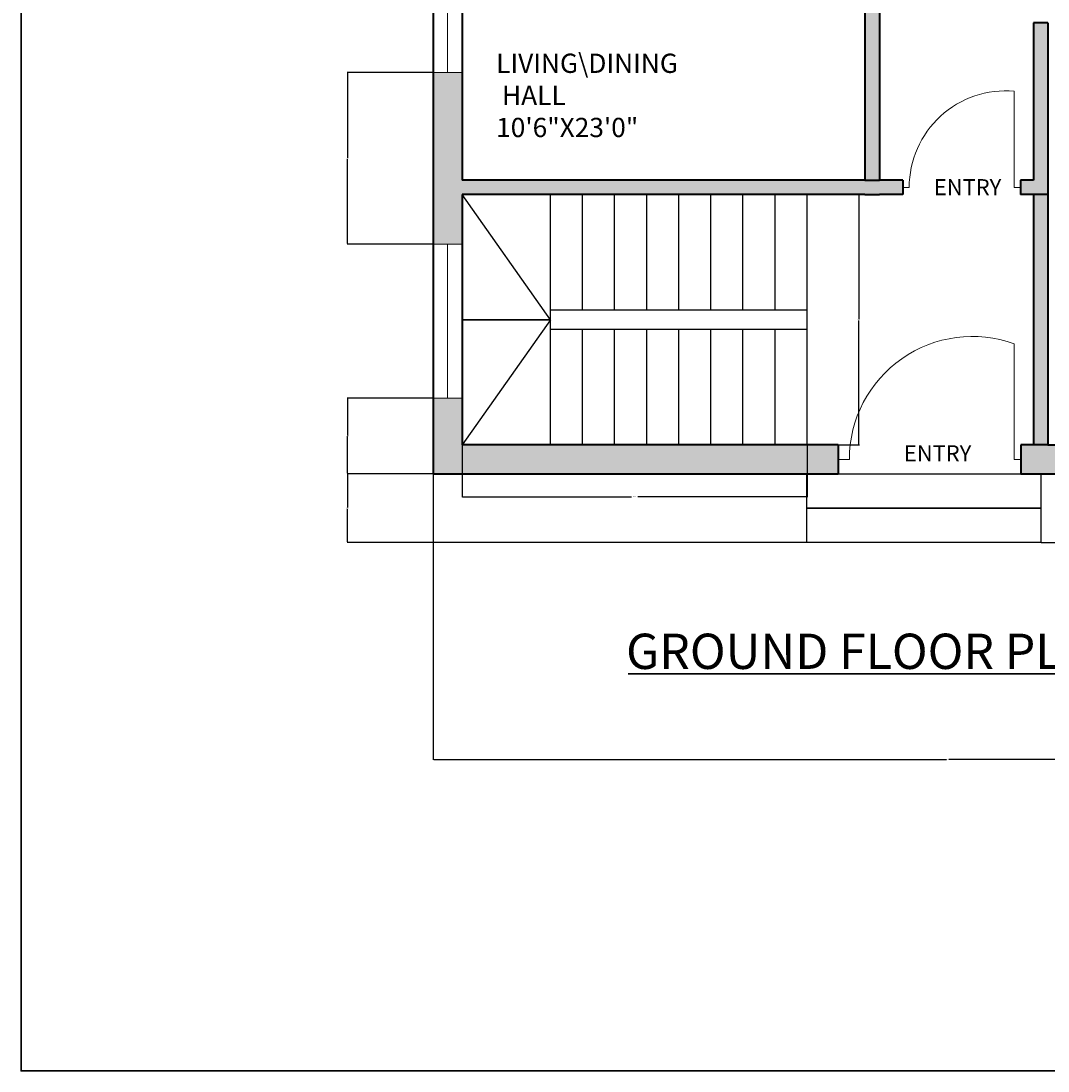
# Model space of a CAD drawing. Units: inches. Extents: x 1441 to 2460, y 1648 to 2683.
# Tile 1 of 35: x 1441 to 1760, y 1648 to 1975. Entities that reach past the tile are written whole.
import ezdxf

# ---------------------------------------------------------------- set-up
doc = ezdxf.new("R2010")
doc.units = ezdxf.units.IN
for name, color, linetype, lineweight in [('A-ANNO-DIMS', 2, 'Continuous', 18), ('A-ANNO-TEXT', 7, 'Continuous', 18), ('A-ANNO-TITL', 7, 'Continuous', 30), ('A-ANNO-TTLB', 7, 'Continuous', 35), ('A-AREA-IDEN', 7, 'Continuous', 20), ('A-DOOR', 3, 'Continuous', 20), ('A-FLOR-STRS', 7, 'Continuous', 25), ('A-GLAZ', 4, 'Continuous', 18), ('A-WALL', 7, 'Continuous', 40)]:
    doc.layers.add(name, color=color, linetype=linetype, lineweight=lineweight)
doc.layers.add('A-WALL-PATT', color=251, linetype='Continuous', lineweight=13, true_color=0x636466)
doc.styles.get("Standard").update_dxf_attribs({"font": 'arial.ttf'})
doc.dimstyles.get("Standard").update_dxf_attribs({"dimtxt": 0.18, "dimasz": 0.18, "dimexe": 0.18, "dimexo": 0.0625, "dimgap": 0.09, "dimtad": 0, "dimtih": 1, "dimtoh": 1, "dimdec": 4, "dimzin": 0, "dimdsep": 46, "dimtxsty": 'Standard', "dimcen": 0.09, "dimadec": 0, "dimazin": 0, "dimtfac": 1, "dimtdec": 4, "dimtofl": 0, "dimtmove": 0, "dimatfit": 3, "dimfxl": 1, "dimtolj": 1, "dimtzin": 0, "dimarcsym": 0})

# ---------------------------------------------------------------- blocks, each defined once
blk = doc.blocks.new('DOOR-ENTRY-OUTER')
for p, q in [((54.89, 0), (54.89, 36)), ((0, 0), (1.52, 0)), ((1.52, 0), (3.52, 0)), ((56.89, 0), (54.89, 0))]:
    blk.add_line(p, q)
blk.add_arc((41.82, 0), 38.3, 70.0399, 180)
blk = doc.blocks.new('DOOR-ENTRY-INNER')
for p, q in [((34.71, 24.01), (34.71, 30.01)), ((34.71, 0.01), (34.71, 24.01)), ((0, 0.01), (2, 0.01)), ((36.71, 0.01), (34.71, 0.01))]:
    blk.add_line(p, q)
blk.add_arc((32.11, 0.01), 30.11, 85.0485, 180)
blk = doc.blocks.new('WIN-48-SASH')
for p, q in [((9, 48), (4.5, 48)), ((4.5, 48), (4.5, 0)), ((4.5, 0), (0, 0))]:
    blk.add_line(p, q)
blk = doc.blocks.new('STAIR-RETURN-PLAN')
for p, q in [((27.5, 39), (0, 78)), ((27.5, 0), (27.5, 78)), ((37.5, 42), (37.5, 78)), ((47.5, 42), (47.5, 78)), ((57.5, 42), (57.5, 78)), ((67.5, 42), (67.5, 78)), ((77.5, 42), (77.5, 78)), ((87.5, 42), (87.5, 78)), ((97.5, 42), (97.5, 78)), ((107.5, 0), (107.5, 78)), ((107.5, 42), (27.5, 42)), ((27.5, 39), (0, 39)), ((0, 39), (27.5, 39)), ((27.5, 39), (0, 0)), ((107.5, 36), (27.5, 36)), ((37.5, 0), (37.5, 36)), ((47.5, 0), (47.5, 36)), ((57.5, 0), (57.5, 36)), ((67.5, 0), (67.5, 36)), ((77.5, 0), (77.5, 36)), ((87.5, 0), (87.5, 36)), ((97.5, 0), (97.5, 36))]:
    blk.add_line(p, q)
blk = doc.blocks.new('*D40')
at = {"layer": 'A-ANNO-DIMS', "color": 0, "lineweight": -2, "transparency": 16777216}
for p, q in [((1577.89, 1843.13), (1577.89, 1826.89)), ((1685.39, 1843.13), (1685.39, 1826.89)), ((1578.07, 1827.07), (1630.64, 1827.07)), ((1685.21, 1827.07), (1632.64, 1827.07))]:
    blk.add_line(p, q, dxfattribs=at)
at = {"layer": 'A-ANNO-DIMS', "color": 0, "transparency": 16777216}
for points in [[(1578.07, 1827.1), (1578.07, 1827.04), (1577.89, 1827.07)], [(1685.21, 1827.1), (1685.21, 1827.04), (1685.39, 1827.07)]]:
    blk.add_solid(points, dxfattribs=at)
at = {"layer": 'Defpoints', "color": 0, "transparency": 16777216}
for p in [(1577.89, 1843.2), (1685.39, 1843.2), (1685.39, 1827.07)]:
    blk.add_point(p, dxfattribs=at)
at = {"layer": 'A-ANNO-DIMS', "color": 0, "transparency": 16777216, "insert": (1631.64, 1827.07), "char_height": 0.18, "attachment_point": 5}
blk.add_mtext('\\A1;STAIR 108 TYP.', dxfattribs=at)
blk = doc.blocks.new('*D41')
at = {"layer": 'A-ANNO-DIMS', "color": 0, "lineweight": -2, "transparency": 16777216}
for p, q in [((1685.45, 1921.2), (1701.7, 1921.2)), ((1701.52, 1921.02), (1701.52, 1882.38)), ((1701.52, 1843.38), (1701.52, 1882.01)), ((1685.45, 1843.2), (1701.7, 1843.2))]:
    blk.add_line(p, q, dxfattribs=at)
at = {"layer": 'A-ANNO-DIMS', "color": 0, "transparency": 16777216}
for points in [[(1701.49, 1921.02), (1701.55, 1921.02), (1701.52, 1921.2)], [(1701.49, 1843.38), (1701.55, 1843.38), (1701.52, 1843.2)]]:
    blk.add_solid(points, dxfattribs=at)
at = {"layer": 'Defpoints', "color": 0, "transparency": 16777216}
for p in [(1685.39, 1921.2), (1701.52, 1921.2), (1685.39, 1843.2)]:
    blk.add_point(p, dxfattribs=at)
at = {"layer": 'A-ANNO-DIMS', "color": 0, "transparency": 16777216, "insert": (1701.52, 1882.2), "char_height": 0.18, "attachment_point": 5}
blk.add_mtext('\\A1;78 TYP.', dxfattribs=at)
blk = doc.blocks.new('*D66')
at = {"layer": 'A-ANNO-DIMS', "color": 0, "lineweight": -2, "transparency": 16777216}
for p, q in [((1568.89, 1834.13), (1568.89, 1745.01)), ((1889.39, 1834.13), (1889.39, 1745.01)), ((1569.07, 1745.19), (1728.74, 1745.19)), ((1889.21, 1745.19), (1729.53, 1745.19))]:
    blk.add_line(p, q, dxfattribs=at)
at = {"layer": 'A-ANNO-DIMS', "color": 0, "transparency": 16777216}
for points in [[(1569.07, 1745.22), (1569.07, 1745.16), (1568.89, 1745.19)], [(1889.21, 1745.22), (1889.21, 1745.16), (1889.39, 1745.19)]]:
    blk.add_solid(points, dxfattribs=at)
at = {"layer": 'Defpoints', "color": 0, "transparency": 16777216}
for p in [(1568.89, 1834.2), (1889.39, 1834.2), (1889.39, 1745.19)]:
    blk.add_point(p, dxfattribs=at)
at = {"layer": 'A-ANNO-DIMS', "color": 0, "transparency": 16777216, "insert": (1729.14, 1745.19), "char_height": 0.18, "attachment_point": 5}
blk.add_mtext('\\A1;320.5', dxfattribs=at)
blk = doc.blocks.new('*D67')
at = {"layer": 'A-ANNO-DIMS', "color": 0, "lineweight": -2, "transparency": 16777216}
for p, q in [((1889.45, 2298.7), (1916.22, 2298.7)), ((1916.04, 2298.52), (1916.04, 2055.94)), ((1916.04, 1813), (1916.04, 2055.57)), ((1758.22, 1812.82), (1916.22, 1812.82))]:
    blk.add_line(p, q, dxfattribs=at)
at = {"layer": 'A-ANNO-DIMS', "color": 0, "transparency": 16777216}
for points in [[(1916.01, 2298.52), (1916.07, 2298.52), (1916.04, 2298.7)], [(1916.01, 1813), (1916.07, 1813), (1916.04, 1812.82)]]:
    blk.add_solid(points, dxfattribs=at)
at = {"layer": 'Defpoints', "color": 0, "transparency": 16777216}
for p in [(1889.39, 2298.7), (1916.04, 2298.7), (1758.16, 1812.82)]:
    blk.add_point(p, dxfattribs=at)
at = {"layer": 'A-ANNO-DIMS', "color": 0, "transparency": 16777216, "insert": (1916.04, 2055.76), "char_height": 0.18, "attachment_point": 5}
blk.add_mtext('\\A1;485.9', dxfattribs=at)
blk = doc.blocks.new('*D74')
at = {"layer": 'A-ANNO-DIMS', "color": 0, "lineweight": -2, "transparency": 16777216}
for p, q in [((1568.82, 1834.2), (1542.06, 1834.2)), ((1542.24, 1834.02), (1542.24, 1823.69)), ((1542.24, 1813), (1542.24, 1823.32)), ((1685.23, 1812.82), (1542.06, 1812.82))]:
    blk.add_line(p, q, dxfattribs=at)
at = {"layer": 'A-ANNO-DIMS', "color": 0, "transparency": 16777216}
for points in [[(1542.21, 1834.02), (1542.27, 1834.02), (1542.24, 1834.2)], [(1542.21, 1813), (1542.27, 1813), (1542.24, 1812.82)]]:
    blk.add_solid(points, dxfattribs=at)
at = {"layer": 'Defpoints', "color": 0, "transparency": 16777216}
for p in [(1542.24, 1834.2), (1568.89, 1834.2), (1685.29, 1812.82)]:
    blk.add_point(p, dxfattribs=at)
at = {"layer": 'A-ANNO-DIMS', "color": 0, "transparency": 16777216, "insert": (1542.24, 1823.51), "char_height": 0.18, "attachment_point": 5}
blk.add_mtext('\\A1;21.38', dxfattribs=at)
blk = doc.blocks.new('*D75')
at = {"layer": 'A-ANNO-DIMS', "color": 0, "lineweight": -2, "transparency": 16777216}
for p, q in [((1568.82, 1857.79), (1542.06, 1857.79)), ((1542.24, 1857.61), (1542.24, 1846.18)), ((1542.24, 1834.38), (1542.24, 1845.81)), ((1568.82, 1834.2), (1542.06, 1834.2))]:
    blk.add_line(p, q, dxfattribs=at)
at = {"layer": 'A-ANNO-DIMS', "color": 0, "transparency": 16777216}
for points in [[(1542.21, 1857.61), (1542.27, 1857.61), (1542.24, 1857.79)], [(1542.21, 1834.38), (1542.27, 1834.38), (1542.24, 1834.2)]]:
    blk.add_solid(points, dxfattribs=at)
at = {"layer": 'Defpoints', "color": 0, "transparency": 16777216}
for p in [(1542.24, 1857.79), (1568.89, 1857.79), (1568.89, 1834.2)]:
    blk.add_point(p, dxfattribs=at)
at = {"layer": 'A-ANNO-DIMS', "color": 0, "transparency": 16777216, "insert": (1542.24, 1845.99), "char_height": 0.18, "attachment_point": 5}
blk.add_mtext('\\A1;23.596', dxfattribs=at)
blk = doc.blocks.new('*D76')
at = {"layer": 'A-ANNO-DIMS', "color": 0, "lineweight": -2, "transparency": 16777216}
for p, q in [((1568.82, 1959.24), (1542.06, 1959.24)), ((1542.24, 1959.06), (1542.24, 1932.7)), ((1542.24, 1905.97), (1542.24, 1932.33)), ((1568.82, 1905.79), (1542.06, 1905.79))]:
    blk.add_line(p, q, dxfattribs=at)
at = {"layer": 'A-ANNO-DIMS', "color": 0, "transparency": 16777216}
for points in [[(1542.21, 1959.06), (1542.27, 1959.06), (1542.24, 1959.24)], [(1542.21, 1905.97), (1542.27, 1905.97), (1542.24, 1905.79)]]:
    blk.add_solid(points, dxfattribs=at)
at = {"layer": 'Defpoints', "color": 0, "transparency": 16777216}
for p in [(1542.24, 1959.24), (1568.89, 1959.24), (1568.89, 1905.79)]:
    blk.add_point(p, dxfattribs=at)
at = {"layer": 'A-ANNO-DIMS', "color": 0, "transparency": 16777216, "insert": (1542.24, 1932.52), "char_height": 0.18, "attachment_point": 5}
blk.add_mtext('\\A1;53.45', dxfattribs=at)

msp = doc.modelspace()

# ---------------------------------------------------------------- hatches: boundary and pattern name
at = {"layer": 'A-WALL-PATT'}
h = msp.add_hatch(color=256, dxfattribs=at)
h.dxf.hatch_style = 1
h.paths.add_polyline_path([(1627.5085, 2298.6952), (1568.8859, 2298.6952), (1568.8859, 2246.9605), (1577.8859, 2246.9605), (1577.8859, 2289.6952), (1627.5085, 2289.6952), (1627.5085, 2294.1952)])
h.paths.add_polyline_path([(1675.5777, 2298.6952), (1651.5085, 2298.6952), (1651.5085, 2289.6952), (1675.5777, 2289.6952), (1675.5777, 2294.1952)])
h.paths.add_polyline_path([(1667.3859, 2289.6952), (1662.8859, 2289.6952), (1662.8859, 2233.0622), (1667.3859, 2233.0622)])
h.paths.add_polyline_path([(1715.8721, 2294.3362), (1715.8721, 2295.2788), (1715.8721, 2298.6952), (1699.5777, 2298.6952), (1699.5777, 2289.6952), (1715.8721, 2289.6952)])
h.paths.add_polyline_path([(1707.8859, 2289.6952), (1703.3859, 2289.6952), (1703.3859, 2199.6952), (1707.8859, 2199.6952)])
h.paths.add_polyline_path([(1760.3859, 2204.637), (1755.8859, 2204.637), (1755.8859, 2199.6952), (1667.3859, 2199.6952), (1667.3859, 2204.637), (1662.8859, 2204.637), (1662.8859, 2195.1952), (1760.3859, 2195.1952)])
h.paths.add_polyline_path([(1760.3859, 2289.6952), (1755.8859, 2289.6952), (1755.8859, 2233.0622), (1760.3859, 2233.0622)])
h.paths.add_polyline_path([(1889.3859, 2298.6952), (1739.8721, 2298.6952), (1739.8721, 2289.6952), (1880.3859, 2289.6952), (1880.3859, 2250.8051), (1889.3859, 2250.8051)])
h.paths.add_polyline_path([(1889.3859, 2202.8051), (1880.3859, 2202.8051), (1880.3859, 2157.6952), (1747.948, 2157.6952), (1747.948, 2153.1952), (1755.8859, 2153.1952), (1755.8859, 2058.005), (1760.3859, 2058.005), (1760.3859, 2153.1952), (1880.3859, 2153.1952), (1880.3859, 2124.108), (1889.3859, 2124.108)])
h.paths.add_polyline_path([(1889.3859, 1984.8305), (1880.3859, 1984.8305), (1880.3859, 1834.1952), (1889.3859, 1834.1952)])
h.paths.add_polyline_path([(1889.3859, 2076.108), (1880.3859, 2076.108), (1880.3859, 2008.8305), (1889.3859, 2008.8305)])
h.paths.add_polyline_path([(1880.3859, 2027.1952), (1800.8859, 2027.1952), (1800.8859, 2000.9452), (1805.3859, 2000.9452), (1805.3859, 2022.6952), (1880.3859, 2022.6952)])
h.paths.add_polyline_path([(1800.8859, 2027.1952), (1760.3859, 2027.1952), (1760.3859, 2030.7912), (1755.8859, 2030.7912), (1755.8859, 2022.6952), (1800.8859, 2022.6952)])
h.paths.add_polyline_path([(1880.3859, 1974.6952), (1805.3859, 1974.6952), (1805.3859, 1978.7973), (1800.8859, 1978.7973), (1800.8859, 1974.6952), (1794.8823, 1974.6952), (1794.8823, 1970.1952), (1800.8859, 1970.1952), (1805.3859, 1970.1952), (1880.3859, 1970.1952)])
h.paths.add_polyline_path([(1760.3859, 1974.6952), (1755.8859, 1974.6952), (1755.8859, 1925.6952), (1751.8616, 1925.6952), (1751.8616, 1921.1952), (1760.3859, 1921.1952)])
h.paths.add_polyline_path([(1760.3859, 1921.1952), (1755.8859, 1921.1952), (1755.8859, 1843.1952), (1760.3859, 1843.1952)])
h.paths.add_polyline_path([(1799.1136, 1838.6952), (1799.1136, 1843.1952), (1760.3859, 1843.1952), (1751.8944, 1843.1952), (1751.8944, 1834.1952), (1758.1615, 1834.1952), (1799.1136, 1834.1952)])
h.paths.add_polyline_path([(1880.3859, 1843.1952), (1859.1136, 1843.1952), (1859.1136, 1834.1952), (1880.3859, 1834.1952)])
h.paths.add_polyline_path([(1577.8859, 1857.7914), (1568.8859, 1857.7914), (1568.8859, 1834.1952), (1695.0034, 1834.1952), (1695.0034, 1838.6952), (1695.0034, 1843.1952), (1577.8859, 1843.1952)])
h.paths.add_polyline_path([(1577.8859, 1959.2399), (1573.3859, 1959.2399), (1568.8859, 1959.2399), (1568.8859, 1905.7914), (1577.8859, 1905.7914), (1577.8859, 1921.1952), (1703.3859, 1921.1952), (1707.8859, 1921.1952), (1715.1501, 1921.1952), (1715.1501, 1925.6952), (1707.8859, 1925.6952), (1703.3859, 1925.6952), (1577.8859, 1925.6952)])
h.paths.add_polyline_path([(1577.8859, 2106.6907), (1568.8859, 2106.6907), (1568.8859, 2019.2399), (1577.8859, 2019.2399)])
h.paths.add_polyline_path([(1707.8859, 2051.6952), (1703.3859, 2051.6952), (1703.3859, 2048.6952), (1703.3859, 1925.6952), (1707.8859, 1925.6952)])
h.paths.add_polyline_path([(1703.3859, 2051.6952), (1676.3859, 2051.6952), (1676.3859, 2048.6952), (1703.3859, 2048.6952)])
h.paths.add_polyline_path([(1703.3859, 2102.6952), (1676.3859, 2102.6952), (1676.3859, 2099.6952), (1685.3859, 2099.6952), (1703.3859, 2099.6952)])
h.paths.add_polyline_path([(1707.8859, 2153.1952), (1710.5611, 2153.1952), (1710.5611, 2157.6952), (1707.8859, 2157.6952), (1707.8859, 2195.1952), (1703.3859, 2195.1952), (1703.3859, 2099.6952), (1707.8859, 2099.6952)])
h.paths.add_polyline_path([(1577.8859, 2198.9605), (1568.8859, 2198.9605), (1568.8859, 2166.6907), (1577.8859, 2166.6907)])

# ---------------------------------------------------------------- linework, layer by layer
at = {"layer": 'A-ANNO-TITL'}
msp.add_line((1629.5852, 1771.8364), (1798.1081, 1771.8364), dxfattribs=at)
at = {"layer": 'A-ANNO-TTLB'}
msp.add_lwpolyline([(1440.5107, 2682.6413), (2460.193, 2682.6413), (2460.193, 1648.08), (1440.5107, 1648.08)], close=True, dxfattribs=at)
at = {"layer": 'A-DOOR'}
msp.add_line((1695.0034, 1834.1952), (1695.0034, 1838.6952), dxfattribs=at)
at = {"layer": 'A-FLOR-STRS'}
for points in [[(1685.2885, 1834.1952), (1758.1615, 1834.1952), (1758.1615, 1823.5061), (1685.2885, 1823.5061)], [(1685.2885, 1834.1952), (1758.1615, 1834.1952), (1758.1615, 1823.5061), (1685.2885, 1823.5061)], [(1685.2885, 1823.5061), (1758.1615, 1823.5061), (1758.1615, 1812.8171), (1685.2885, 1812.8171)]]:
    msp.add_lwpolyline(points, close=True, dxfattribs=at)
at = {"layer": 'A-GLAZ'}
for p, q in [((1573.3859, 1959.2399), (1573.3859, 2019.2399)), ((1568.8859, 1959.2399), (1577.8859, 1959.2399)), ((1577.8859, 1959.2399), (1573.3859, 1959.2399)), ((1568.8859, 1905.7914), (1577.8859, 1905.7914)), ((1568.8859, 1857.7914), (1577.8859, 1857.7914))]:
    msp.add_line(p, q, dxfattribs=at)
at = {"layer": 'A-WALL'}
for p, q in [((1568.8859, 2298.6952), (1568.8859, 1834.1952)), ((1577.8859, 2289.6952), (1577.8859, 1925.6952)), ((1703.3859, 2051.6952), (1703.3859, 1925.6952)), ((1707.8859, 2051.6952), (1707.8859, 1925.6952)), ((1755.8859, 1974.6952), (1755.8859, 1925.6952)), ((1760.3859, 1974.6952), (1755.8859, 1974.6952)), ((1760.3859, 1974.6952), (1760.3859, 1843.1952)), ((1703.3859, 1925.6952), (1577.8859, 1925.6952)), ((1703.3859, 1925.6952), (1707.8859, 1925.6952)), ((1715.1501, 1925.6952), (1707.8859, 1925.6952)), ((1715.1501, 1925.6952), (1715.1501, 1921.1952)), ((1755.8859, 1925.6952), (1751.8616, 1925.6952)), ((1751.8616, 1925.6952), (1751.8616, 1921.1952)), ((1703.3859, 1921.1952), (1577.8859, 1921.1952)), ((1577.8859, 1921.1952), (1577.8859, 1843.1952)), ((1703.3859, 1921.1952), (1707.8859, 1921.1952)), ((1715.1501, 1921.1952), (1707.8859, 1921.1952)), ((1760.3859, 1921.1952), (1751.8616, 1921.1952)), ((1755.8859, 1921.1952), (1755.8859, 1843.1952)), ((1695.0034, 1843.1952), (1577.8859, 1843.1952)), ((1695.0034, 1843.1952), (1695.0034, 1834.1952)), ((1760.3859, 1843.1952), (1751.8944, 1843.1952)), ((1751.8944, 1843.1952), (1751.8944, 1834.1952)), ((1760.3859, 1843.1952), (1880.3859, 1843.1952)), ((1568.8859, 1834.1952), (1695.0034, 1834.1952)), ((1751.8944, 1834.1952), (1880.3859, 1834.1952))]:
    msp.add_line(p, q, dxfattribs=at)

# ---------------------------------------------------------------- block references
at = {"layer": 'A-DOOR'}
for name, p in [('DOOR-ENTRY-INNER', (1715.15, 1923.44)), ('DOOR-ENTRY-OUTER', (1695, 1838.7))]:
    msp.add_blockref(name, p, dxfattribs=at)
at = {"layer": 'A-FLOR-STRS'}
msp.add_blockref('STAIR-RETURN-PLAN', (1577.89, 1843.2), dxfattribs=at)
at = {"layer": 'A-GLAZ'}
msp.add_blockref('WIN-48-SASH', (1568.89, 1857.7909), dxfattribs=at)

# ---------------------------------------------------------------- texts
at = {"layer": 'A-ANNO-TEXT', "char_height": 5, "attachment_point": 1}
for insert in [(1724.8512, 1926.0225), (1715.5089, 1843.0822)]:
    msp.add_mtext_dynamic_manual_height_columns('ENTRY', width=85.554017, gutter_width=12.5, heights=[0], dxfattribs=dict(at, insert=insert))
at = {"layer": 'A-ANNO-TITL', "insert": (1628.9764, 1784.3785), "char_height": 11, "attachment_point": 1}
msp.add_mtext_dynamic_manual_height_columns('GROUND FLOOR PLAN', width=244.599836, gutter_width=12.5, heights=[0], dxfattribs=at)
at = {"layer": 'A-AREA-IDEN', "insert": (1588.508, 1965.133), "char_height": 6, "attachment_point": 1}
msp.add_mtext_dynamic_manual_height_columns('LIVING\\\\DINING\\P HALL\\P10\'6"X23\'0"', width=85.554017, gutter_width=12.5, heights=[0], dxfattribs=at)

# ---------------------------------------------------------------- dimensions: what is measured, and where the dimension line sits
at = {"layer": 'A-ANNO-DIMS'}
for base, p1, p2, override, picture, middle in [((1916.0359, 2298.6952), (1758.1615, 1812.8171), (1889.3859, 2298.6952), {"dimdec": 1, "dimlfac": 1, "dimrnd": 0, "dimzin": 0, "dimdsep": 46, "dimlunit": 2}, '*D67', (1916.0359, 2055.7561)), ((1542.2359, 1959.2399), (1568.8859, 1905.7914), (1568.8859, 1959.2399), {"dimdec": 2, "dimlfac": 1, "dimrnd": 0, "dimzin": 0, "dimdsep": 46, "dimlunit": 2}, '*D76', (1542.2359, 1932.5157)), ((1542.2359, 1857.7914), (1568.8859, 1834.1952), (1568.8859, 1857.7914), {"dimdec": 3, "dimlfac": 1, "dimrnd": 0, "dimzin": 0, "dimdsep": 46, "dimlunit": 2}, '*D75', (1542.2359, 1845.9933)), ((1542.2359, 1834.1952), (1685.2885, 1812.8171), (1568.8859, 1834.1952), {"dimdec": 2, "dimlfac": 1, "dimrnd": 0, "dimzin": 0, "dimdsep": 46, "dimlunit": 2}, '*D74', (1542.2359, 1823.5061))]:
    dim = msp.add_linear_dim(base=base, p1=p1, p2=p2, angle=90, dimstyle='Standard', override=override, dxfattribs=at)
    dim.commit()
    dim.dimension.update_dxf_attribs({"geometry": picture, "text_midpoint": middle})
dim = msp.add_linear_dim(base=(1701.5154, 1921.1952), p1=(1685.3898, 1843.1952), p2=(1685.3898, 1921.1952), angle=90, text='<> TYP.', dimstyle='Standard', override={"dimdec": 0, "dimlfac": 1, "dimrnd": 0, "dimzin": 0, "dimdsep": 46, "dimlunit": 2}, dxfattribs=at)
dim.commit()
dim.dimension.update_dxf_attribs({"geometry": '*D41', "text_midpoint": (1701.5154, 1882.1952)})
dim = msp.add_linear_dim(base=(1685.3898, 1827.0696), p1=(1577.8859, 1843.1952), p2=(1685.3898, 1843.1952), text='STAIR <> TYP.', dimstyle='Standard', override={"dimdec": 0, "dimlfac": 1, "dimrnd": 0, "dimzin": 0, "dimdsep": 46, "dimlunit": 2}, dxfattribs=at)
dim.commit()
dim.dimension.update_dxf_attribs({"geometry": '*D40', "text_midpoint": (1631.6379, 1827.0696)})
dim = msp.add_linear_dim(base=(1889.3859, 1745.1864), p1=(1568.8859, 1834.1952), p2=(1889.3859, 1834.1952), dimstyle='Standard', override={"dimdec": 1, "dimlfac": 1, "dimrnd": 0, "dimzin": 0, "dimdsep": 46, "dimlunit": 2}, dxfattribs=at)
dim.commit()
dim.dimension.update_dxf_attribs({"geometry": '*D66', "text_midpoint": (1729.1359, 1745.1864)})

doc.saveas('drawing.dxf')
